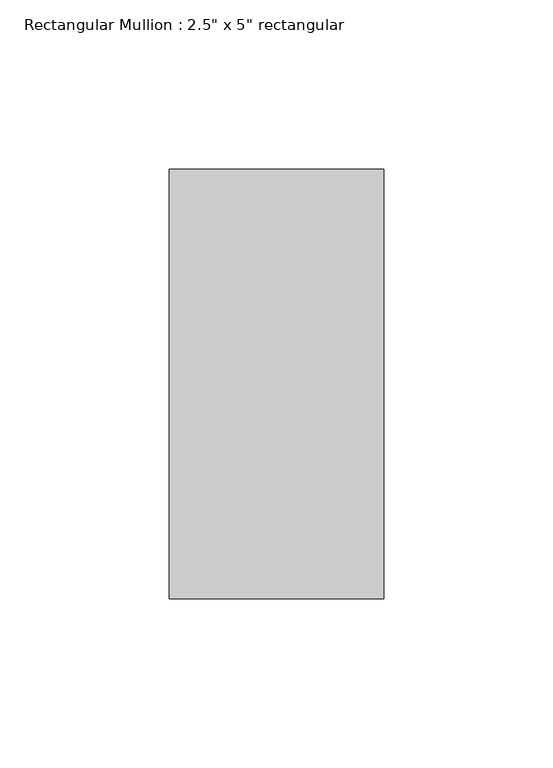
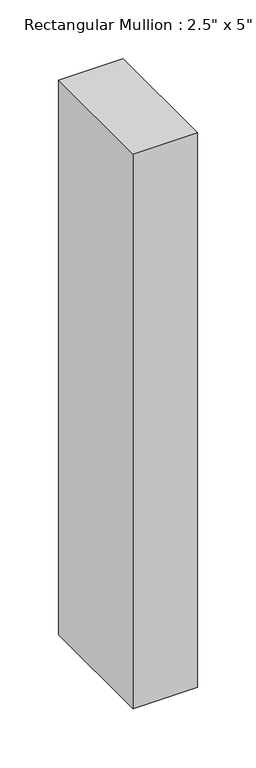
"""IFC4 building model written with IfcOpenShell, lengths in millimetres: member geometry."""

from ifc_helpers import new_model, si_unit, frame, origin, place, context, project, spatial, polyline, outline, extrude, source, transform, mapped, element, save


def member_830eb86c(model_context):
    return source(origin(), model_context, "Body", "SweptSolid", [
        extrude(outline(polyline([(0.0, 63.5), (0.0, -63.5), (-63.5, -63.5), (-63.5, 63.5), (0.0, 63.5)])), frame((0.0, 0.0, -577.85), z_axis=(0.0, 0.0, 1.0), x_axis=(1.0, 0.0, 0.0)), (0.0, 0.0, 1.0), 577.85),
    ])


if __name__ == "__main__":
    model = new_model("IFC4")
    model_context = context("Model", 3, world=origin())
    ifc_project = project(units=[si_unit("LENGTHUNIT", "METRE", prefix="MILLI")], contexts=[model_context])
    site = spatial("IfcSite", under=ifc_project)
    building = spatial("IfcBuilding", under=site)
    placement = place(None, origin())
    member_shape = member_830eb86c(model_context)
    element("IfcMember", 1, ObjectType="Rectangular Mullion : 2.5\" x 5\" rectangular", at=placement, inside=building, context=model_context, shape_type="MappedRepresentation", body=[
        mapped(member_shape, transform((0.0, 0.0, 0.0), x_axis=(1.0, 0.0, 0.0), y_axis=(0.0, 1.0, 0.0), z_axis=(0.0, 0.0, 1.0))),
    ])
    save(model, "model.ifc")

# Revit data of these elements
# Type "Rectangular Mullion : 2.5\" x 5\" rectangular"
#   built-in parameter 1007304 = 0.416667 (stored number, unit not read)
#   built-in parameter 1007301 = 0.104167 (stored number, unit not read)
#   built-in parameter 1007300 = 0.104167 (stored number, unit not read)
